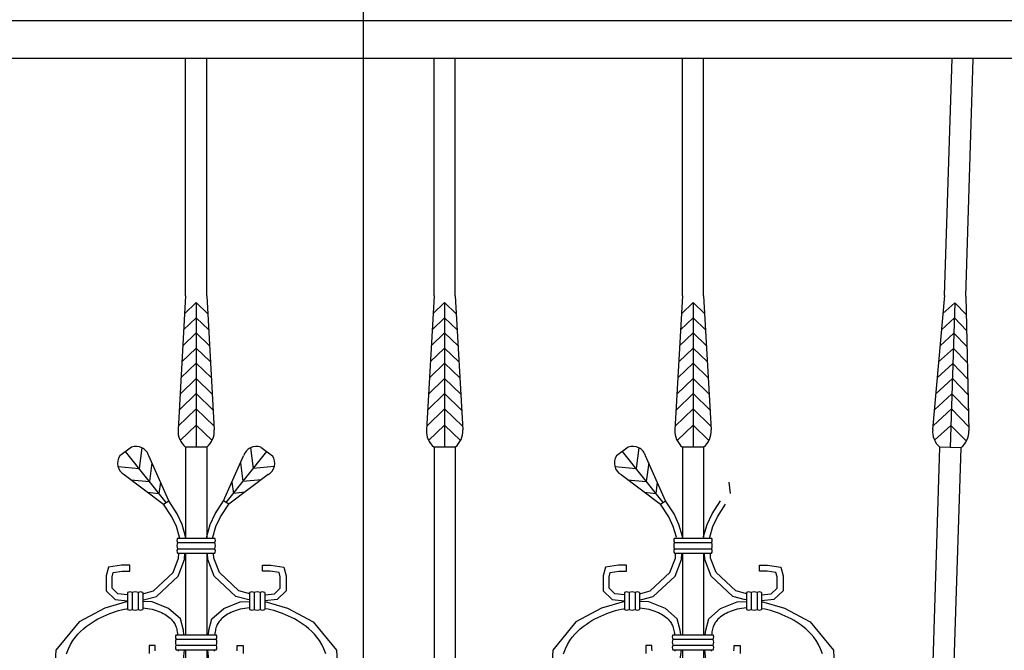
# Model space of a CAD drawing. Units: inches. Extents: x 2278 to 7495, y -71 to 1198.
# Tile 20 of 44: x 5007 to 5033, y 143 to 160. Entities that reach past the tile are written whole.
import ezdxf

# ---------------------------------------------------------------- set-up
doc = ezdxf.new("R2010")
doc.units = ezdxf.units.IN
doc.header["$MEASUREMENT"] = 0
doc.layers.add('A-ANNO-DIMS', color=2, linetype='Continuous', lineweight=18)
doc.layers.add('A-ELEV', color=7, linetype='Continuous', lineweight=25)
doc.styles.get("Standard").update_dxf_attribs({"font": 'arial.ttf'})
doc.dimstyles.get("Standard").update_dxf_attribs({"dimtxt": 6, "dimasz": 3, "dimexe": 0.18, "dimexo": 0.0625, "dimgap": 0.09, "dimtad": 0, "dimtih": 1, "dimtoh": 1, "dimdec": 0, "dimzin": 0, "dimdsep": 46, "dimlunit": 3, "dimtxsty": 'Standard', "dimblk": 'ARCHTICK', "dimcen": 0.09, "dimadec": 0, "dimazin": 0, "dimtfac": 1, "dimtdec": 0, "dimtofl": 0, "dimtmove": 0, "dimatfit": 3, "dimfxl": 1, "dimtolj": 1, "dimtzin": 0, "dimarcsym": 0})

# ---------------------------------------------------------------- blocks, each defined once
blk = doc.blocks.new('BALUSTER-ORNATE-A')
for p, q in [((3.585, 26.003), (3.585, 32.384)), ((4.155, 26.003), (4.155, 32.38)), ((3.585, 26.003), (3.383, 22.393)), ((4.155, 26.003), (4.357, 22.393)), ((3.558, 25.516), (3.87, 25.818)), ((3.87, 25.818), (3.87, 21.929)), ((4.182, 25.516), (3.87, 25.818)), ((3.533, 25.084), (3.87, 25.41)), ((4.207, 25.084), (3.87, 25.41)), ((3.509, 24.653), (3.87, 25.001)), ((4.231, 24.653), (3.87, 25.001)), ((3.485, 24.221), (3.87, 24.593)), ((4.255, 24.221), (3.87, 24.593)), ((3.461, 23.79), (3.87, 24.185)), ((4.279, 23.79), (3.87, 24.185)), ((3.437, 23.358), (3.87, 23.777)), ((4.303, 23.358), (3.87, 23.777)), ((3.413, 22.927), (3.87, 23.369)), ((4.327, 22.927), (3.87, 23.369)), ((3.388, 22.495), (3.87, 22.961)), ((4.352, 22.495), (3.87, 22.961)), ((3.442, 22.106), (3.87, 22.52)), ((4.299, 22.106), (3.87, 22.52)), ((2.128, 21.929), (1.813, 21.699)), ((3.063, 20.442), (1.97, 21.814)), ((2.412, 21.914), (2.339, 21.352)), ((3.585, 21.929), (3.585, 19.485)), ((4.155, 21.929), (3.585, 21.929)), ((4.155, 21.929), (4.155, 19.485)), ((4.677, 20.442), (5.77, 21.814)), ((5.328, 21.914), (5.401, 21.352)), ((5.612, 21.929), (5.927, 21.699)), ((3.131, 20.487), (2.594, 21.696)), ((2.678, 21.507), (2.613, 21.007)), ((4.609, 20.487), (5.146, 21.696)), ((5.062, 21.507), (5.127, 21.007)), ((1.774, 21.406), (2.339, 21.352)), ((1.936, 21.192), (2.995, 20.398)), ((5.804, 21.192), (4.745, 20.398)), ((5.966, 21.406), (5.401, 21.352)), ((2.111, 21.055), (2.613, 21.007)), ((2.907, 20.992), (2.868, 20.688)), ((4.833, 20.992), (4.872, 20.688)), ((5.629, 21.055), (5.127, 21.007)), ((2.562, 20.717), (2.868, 20.688)), ((5.178, 20.717), (4.872, 20.688)), ((2.995, 20.398), (3.131, 20.487)), ((3.217, 20.057), (2.995, 20.398)), ((3.36, 20.135), (3.131, 20.487)), ((4.38, 20.135), (4.609, 20.487)), ((4.523, 20.057), (4.745, 20.398)), ((4.745, 20.398), (4.609, 20.487)), ((3.49, 19.852), (3.36, 20.135)), ((4.25, 19.852), (4.38, 20.135)), ((3.337, 19.795), (3.217, 20.057)), ((4.403, 19.795), (4.523, 20.057)), ((3.421, 19.506), (3.337, 19.795)), ((3.585, 19.526), (3.49, 19.852)), ((4.155, 19.526), (4.25, 19.852)), ((4.319, 19.506), (4.403, 19.795)), ((3.37, 19.485), (4.37, 19.485)), ((3.37, 19.363), (4.37, 19.363)), ((3.42, 19.485), (3.421, 19.506)), ((3.583, 19.485), (3.585, 19.526)), ((4.157, 19.485), (4.155, 19.526)), ((4.32, 19.485), (4.319, 19.506)), ((3.37, 19.2), (4.37, 19.2)), ((3.37, 19.077), (4.37, 19.077)), ((3.396, 18.942), (3.402, 19.077)), ((3.558, 18.908), (3.565, 19.077)), ((3.585, 19.077), (3.585, 16.887)), ((4.155, 19.077), (4.155, 16.887)), ((4.182, 18.908), (4.175, 19.077)), ((4.344, 18.942), (4.338, 19.077)), ((3.247, 18.557), (3.396, 18.942)), ((3.385, 18.463), (3.558, 18.908)), ((4.355, 18.463), (4.182, 18.908)), ((4.493, 18.557), (4.344, 18.942)), ((1.513, 18.705), (1.449, 18.469)), ((1.866, 18.759), (1.513, 18.705)), ((1.612, 18.447), (1.642, 18.56)), ((1.642, 18.56), (1.879, 18.596)), ((2.084, 18.759), (1.866, 18.759)), ((1.879, 18.596), (2.084, 18.596)), ((2.084, 18.596), (2.084, 18.759)), ((2.719, 18.062), (3.247, 18.557)), ((5.021, 18.062), (4.493, 18.557)), ((5.656, 18.596), (5.656, 18.759)), ((5.656, 18.759), (5.874, 18.759)), ((5.861, 18.596), (5.656, 18.596)), ((6.098, 18.56), (5.861, 18.596)), ((5.874, 18.759), (6.227, 18.705)), ((6.128, 18.447), (6.098, 18.56)), ((6.227, 18.705), (6.291, 18.469)), ((1.449, 18.469), (1.449, 18.069)), ((1.612, 18.138), (1.612, 18.447)), ((2.801, 17.915), (3.385, 18.463)), ((4.939, 17.915), (4.355, 18.463)), ((6.128, 18.138), (6.128, 18.447)), ((6.291, 18.469), (6.291, 18.069)), ((1.449, 18.069), (1.694, 17.833)), ((1.767, 17.989), (1.612, 18.138)), ((2.026, 18.021), (2.026, 17.565)), ((2.148, 18.021), (2.148, 17.565)), ((2.311, 18.021), (2.311, 17.565)), ((2.434, 18.021), (2.434, 17.565)), ((2.462, 17.993), (2.719, 18.062)), ((5.278, 17.993), (5.021, 18.062)), ((5.306, 18.021), (5.306, 17.565)), ((5.429, 18.021), (5.429, 17.565)), ((5.592, 18.021), (5.592, 17.565)), ((5.714, 18.021), (5.714, 17.565)), ((5.973, 17.989), (6.128, 18.138)), ((6.291, 18.069), (6.046, 17.833)), ((2.026, 17.782), (1.412, 17.603)), ((1.694, 17.833), (2.026, 17.797)), ((2.026, 17.961), (1.767, 17.989)), ((2.434, 17.99), (2.462, 17.993)), ((2.434, 17.826), (2.492, 17.833)), ((2.683, 17.766), (2.434, 17.777)), ((2.492, 17.833), (2.801, 17.915)), ((3.128, 17.594), (2.683, 17.766)), ((4.612, 17.594), (5.057, 17.766)), ((5.248, 17.833), (4.939, 17.915)), ((5.057, 17.766), (5.306, 17.777)), ((5.306, 17.826), (5.248, 17.833)), ((5.306, 17.99), (5.278, 17.993)), ((5.714, 17.961), (5.973, 17.989)), ((6.046, 17.833), (5.714, 17.797)), ((5.714, 17.782), (6.328, 17.603)), ((1.412, 17.603), (0.722, 17.231)), ((1.549, 17.454), (1.627, 17.484)), ((1.627, 17.484), (1.705, 17.51)), ((1.705, 17.51), (1.782, 17.533)), ((1.782, 17.533), (1.858, 17.553)), ((1.858, 17.553), (1.933, 17.571)), ((1.933, 17.571), (2.007, 17.585)), ((2.007, 17.585), (2.026, 17.587)), ((2.434, 17.606), (2.499, 17.6)), ((2.499, 17.6), (2.563, 17.592)), ((2.563, 17.592), (2.624, 17.582)), ((2.624, 17.582), (2.683, 17.57)), ((2.683, 17.57), (2.739, 17.556)), ((2.739, 17.556), (2.792, 17.54)), ((2.792, 17.54), (2.843, 17.522)), ((2.843, 17.522), (2.891, 17.503)), ((2.891, 17.503), (2.937, 17.482)), ((2.937, 17.482), (2.981, 17.46)), ((3.446, 17.313), (3.128, 17.594)), ((4.294, 17.313), (4.612, 17.594)), ((4.803, 17.482), (4.759, 17.46)), ((4.849, 17.503), (4.803, 17.482)), ((4.897, 17.522), (4.849, 17.503)), ((4.948, 17.54), (4.897, 17.522)), ((5.001, 17.556), (4.948, 17.54)), ((5.057, 17.57), (5.001, 17.556)), ((5.116, 17.582), (5.057, 17.57)), ((5.177, 17.592), (5.116, 17.582)), ((5.241, 17.6), (5.177, 17.592)), ((5.306, 17.606), (5.241, 17.6)), ((5.733, 17.585), (5.714, 17.587)), ((5.807, 17.571), (5.733, 17.585)), ((5.882, 17.553), (5.807, 17.571)), ((5.958, 17.533), (5.882, 17.553)), ((6.035, 17.51), (5.958, 17.533)), ((6.113, 17.484), (6.035, 17.51)), ((6.191, 17.454), (6.113, 17.484)), ((6.328, 17.603), (7.018, 17.231)), ((0.722, 17.231), (0.096, 16.469)), ((0.993, 17.163), (1.071, 17.216)), ((1.071, 17.216), (1.15, 17.265)), ((1.15, 17.265), (1.23, 17.309)), ((1.23, 17.309), (1.309, 17.35)), ((1.309, 17.35), (1.389, 17.388)), ((1.389, 17.388), (1.469, 17.422)), ((1.469, 17.422), (1.549, 17.454)), ((2.981, 17.46), (3.024, 17.436)), ((3.024, 17.436), (3.064, 17.41)), ((3.064, 17.41), (3.102, 17.384)), ((3.102, 17.384), (3.138, 17.357)), ((3.138, 17.357), (3.171, 17.329)), ((3.171, 17.329), (3.201, 17.301)), ((3.201, 17.301), (3.228, 17.272)), ((3.228, 17.272), (3.252, 17.244)), ((3.252, 17.244), (3.272, 17.217)), ((3.272, 17.217), (3.288, 17.19)), ((3.528, 17.004), (3.446, 17.313)), ((4.212, 17.004), (4.294, 17.313)), ((4.468, 17.217), (4.452, 17.19)), ((4.489, 17.244), (4.468, 17.217)), ((4.512, 17.272), (4.489, 17.244)), ((4.539, 17.301), (4.512, 17.272)), ((4.569, 17.329), (4.539, 17.301)), ((4.602, 17.357), (4.569, 17.329)), ((4.638, 17.384), (4.602, 17.357)), ((4.676, 17.41), (4.638, 17.384)), ((4.716, 17.436), (4.676, 17.41)), ((4.759, 17.46), (4.716, 17.436)), ((6.271, 17.422), (6.191, 17.454)), ((6.351, 17.388), (6.271, 17.422)), ((6.431, 17.35), (6.351, 17.388)), ((6.51, 17.309), (6.431, 17.35)), ((6.59, 17.265), (6.51, 17.309)), ((6.669, 17.216), (6.59, 17.265)), ((6.747, 17.163), (6.669, 17.216)), ((7.018, 17.231), (7.644, 16.469)), ((0.692, 16.9), (0.764, 16.975)), ((0.764, 16.975), (0.839, 17.043)), ((0.839, 17.043), (0.916, 17.105)), ((0.916, 17.105), (0.993, 17.163)), ((3.288, 17.19), (3.303, 17.162)), ((3.303, 17.162), (3.316, 17.134)), ((3.316, 17.134), (3.327, 17.104)), ((3.327, 17.104), (3.337, 17.072)), ((3.337, 17.072), (3.346, 17.038)), ((3.346, 17.038), (3.354, 17.001)), ((3.354, 17.001), (3.361, 16.962)), ((3.361, 16.962), (3.368, 16.922)), ((3.542, 16.887), (3.528, 17.004)), ((4.198, 16.887), (4.212, 17.004)), ((4.379, 16.962), (4.372, 16.922)), ((4.386, 17.001), (4.379, 16.962)), ((4.394, 17.038), (4.386, 17.001)), ((4.403, 17.072), (4.394, 17.038)), ((4.413, 17.104), (4.403, 17.072)), ((4.424, 17.134), (4.413, 17.104)), ((4.437, 17.162), (4.424, 17.134)), ((4.452, 17.19), (4.437, 17.162)), ((6.824, 17.105), (6.747, 17.163)), ((6.901, 17.043), (6.824, 17.105)), ((6.976, 16.975), (6.901, 17.043)), ((7.048, 16.9), (6.976, 16.975)), ((0.495, 16.624), (0.557, 16.727)), ((0.557, 16.727), (0.623, 16.819)), ((0.623, 16.819), (0.692, 16.9)), ((3.329, 16.887), (4.411, 16.887)), ((3.329, 16.764), (4.411, 16.764)), ((3.368, 16.922), (3.374, 16.887)), ((4.372, 16.922), (4.366, 16.887)), ((7.117, 16.819), (7.048, 16.9)), ((7.183, 16.727), (7.117, 16.819)), ((7.245, 16.624), (7.183, 16.727)), ((0.096, 16.469), (0.025, 15.162)), ((0.386, 16.376), (0.438, 16.508)), ((0.438, 16.508), (0.495, 16.624)), ((2.764, 16.599), (2.602, 16.596)), ((2.602, 16.596), (2.602, 16.378)), ((2.766, 16.522), (2.764, 16.599)), ((2.769, 16.452), (2.766, 16.522)), ((3.329, 16.601), (4.411, 16.601)), ((3.329, 16.479), (4.411, 16.479)), ((3.388, 16.479), (3.383, 16.441)), ((3.528, 16.206), (3.557, 16.479)), ((3.585, 16.479), (3.585, 12.578)), ((4.155, 16.479), (4.155, 12.578)), ((4.212, 16.206), (4.183, 16.479)), ((4.352, 16.479), (4.357, 16.441)), ((4.971, 16.452), (4.974, 16.522)), ((4.974, 16.522), (4.976, 16.599)), ((4.976, 16.599), (5.138, 16.596)), ((5.138, 16.596), (5.138, 16.378)), ((7.302, 16.508), (7.245, 16.624)), ((7.354, 16.376), (7.302, 16.508)), ((7.644, 16.469), (7.715, 15.162))]:
    blk.add_line(p, q)
for centre, radius, start, end in [((3.929, 22.355), 0.547, 176.0178, 231.0717), ((3.811, 22.355), 0.547, 308.9283, 3.9822), ((2.253, 21.595), 0.356, 16.4025, 110.5063), ((5.487, 21.595), 0.356, 69.4937, 163.5975), ((2.111, 21.502), 0.356, 146.575, 240.6788), ((5.629, 21.502), 0.356, 299.3212, 33.425), ((3.475, 19.424), 0.121, 149.7768, 210.2232), ((3.563, 19.281), 0.209, 157.1017, 202.8983), ((4.265, 19.424), 0.121, 329.7768, 30.2232), ((4.177, 19.281), 0.209, 337.1017, 22.8983), ((3.475, 19.139), 0.121, 149.7768, 210.2232), ((4.265, 19.139), 0.121, 329.7768, 30.2232), ((2.087, 17.916), 0.121, 59.7768, 120.2232), ((2.23, 17.828), 0.209, 67.1017, 112.8983), ((2.373, 17.916), 0.121, 59.7768, 120.2232), ((5.368, 17.916), 0.121, 59.7768, 120.2232), ((5.51, 17.828), 0.209, 67.1017, 112.8983), ((5.653, 17.916), 0.121, 59.7768, 120.2232), ((2.087, 17.67), 0.121, 239.7768, 300.2232), ((2.23, 17.758), 0.209, 247.1017, 292.8983), ((2.373, 17.67), 0.121, 239.7768, 300.2232), ((5.368, 17.67), 0.121, 239.7768, 300.2232), ((5.51, 17.758), 0.209, 247.1017, 292.8983), ((5.653, 17.67), 0.121, 239.7768, 300.2232), ((3.434, 16.825), 0.121, 149.7768, 210.2232), ((3.522, 16.683), 0.209, 157.1017, 202.8983), ((4.306, 16.825), 0.121, 329.7768, 30.2232), ((4.218, 16.683), 0.209, 337.1017, 22.8983), ((3.434, 16.54), 0.121, 149.7768, 210.2232), ((4.306, 16.54), 0.121, 329.7768, 30.2232)]:
    blk.add_arc(centre, radius, start, end)
blk = doc.blocks.new('BALUSTER-ORNATE-B')
for p, q in [((3.585, 26.003), (3.585, 32.384)), ((4.155, 26.003), (4.155, 32.38)), ((3.585, 26.003), (3.383, 22.393)), ((4.155, 26.003), (4.358, 22.393)), ((3.558, 25.516), (3.87, 25.818)), ((3.87, 25.818), (3.87, 21.929)), ((4.183, 25.516), (3.87, 25.818)), ((3.534, 25.084), (3.87, 25.41)), ((4.207, 25.084), (3.87, 25.41)), ((3.51, 24.653), (3.87, 25.001)), ((4.231, 24.653), (3.87, 25.001)), ((3.485, 24.221), (3.87, 24.593)), ((4.255, 24.221), (3.87, 24.593)), ((3.461, 23.79), (3.87, 24.185)), ((4.279, 23.79), (3.87, 24.185)), ((3.437, 23.358), (3.87, 23.777)), ((4.304, 23.358), (3.87, 23.777)), ((3.413, 22.927), (3.87, 23.369)), ((4.328, 22.927), (3.87, 23.369)), ((3.389, 22.495), (3.87, 22.961)), ((4.352, 22.495), (3.87, 22.961)), ((3.442, 22.106), (3.87, 22.52)), ((4.299, 22.106), (3.87, 22.52)), ((2.128, 21.929), (1.814, 21.699)), ((3.063, 20.442), (1.971, 21.814)), ((2.412, 21.914), (2.339, 21.352)), ((3.585, 21.929), (3.585, 19.485)), ((4.155, 21.929), (3.585, 21.929)), ((4.155, 21.929), (4.155, 19.485)), ((3.132, 20.487), (2.595, 21.696)), ((2.679, 21.507), (2.614, 21.007)), ((1.774, 21.406), (2.339, 21.352)), ((1.936, 21.192), (2.995, 20.398)), ((2.112, 21.055), (2.614, 21.007)), ((2.907, 20.992), (2.868, 20.688)), ((4.833, 20.992), (4.873, 20.688)), ((2.563, 20.717), (2.868, 20.688)), ((2.995, 20.398), (3.132, 20.487)), ((3.217, 20.057), (2.995, 20.398)), ((3.36, 20.135), (3.132, 20.487)), ((4.381, 20.135), (4.609, 20.487)), ((4.524, 20.057), (4.746, 20.398)), ((3.49, 19.852), (3.36, 20.135)), ((4.251, 19.852), (4.381, 20.135)), ((3.337, 19.795), (3.217, 20.057)), ((4.404, 19.795), (4.524, 20.057)), ((3.421, 19.506), (3.337, 19.795)), ((3.585, 19.526), (3.49, 19.852)), ((4.155, 19.526), (4.251, 19.852)), ((4.319, 19.506), (4.404, 19.795)), ((3.37, 19.485), (4.37, 19.485)), ((3.37, 19.363), (4.37, 19.363)), ((3.42, 19.485), (3.421, 19.506)), ((3.583, 19.485), (3.585, 19.526)), ((4.157, 19.485), (4.155, 19.526)), ((4.32, 19.485), (4.319, 19.506)), ((3.37, 19.2), (4.37, 19.2)), ((3.37, 19.077), (4.37, 19.077)), ((3.396, 18.942), (3.402, 19.077)), ((3.558, 18.908), (3.565, 19.077)), ((3.585, 19.077), (3.585, 16.887)), ((4.155, 19.077), (4.155, 16.887)), ((4.183, 18.908), (4.175, 19.077)), ((4.344, 18.942), (4.338, 19.077)), ((3.247, 18.557), (3.396, 18.942)), ((3.386, 18.463), (3.558, 18.908)), ((4.355, 18.463), (4.183, 18.908)), ((4.494, 18.557), (4.344, 18.942)), ((1.513, 18.705), (1.449, 18.469)), ((1.867, 18.759), (1.513, 18.705)), ((1.612, 18.447), (1.643, 18.56)), ((1.643, 18.56), (1.879, 18.596)), ((2.084, 18.759), (1.867, 18.759)), ((1.879, 18.596), (2.084, 18.596)), ((2.084, 18.596), (2.084, 18.759)), ((2.72, 18.062), (3.247, 18.557)), ((5.021, 18.062), (4.494, 18.557)), ((5.656, 18.596), (5.656, 18.759)), ((5.656, 18.759), (5.874, 18.759)), ((5.861, 18.596), (5.656, 18.596)), ((6.098, 18.56), (5.861, 18.596)), ((5.874, 18.759), (6.228, 18.705)), ((6.128, 18.447), (6.098, 18.56)), ((6.228, 18.705), (6.291, 18.469)), ((1.449, 18.469), (1.449, 18.069)), ((1.612, 18.138), (1.612, 18.447)), ((2.801, 17.915), (3.386, 18.463)), ((4.939, 17.915), (4.355, 18.463)), ((6.128, 18.138), (6.128, 18.447)), ((6.291, 18.469), (6.291, 18.069)), ((1.449, 18.069), (1.694, 17.833)), ((1.767, 17.989), (1.612, 18.138)), ((2.027, 18.021), (2.027, 17.565)), ((2.149, 18.021), (2.149, 17.565)), ((2.312, 18.021), (2.312, 17.565)), ((2.434, 18.021), (2.434, 17.565)), ((2.462, 17.993), (2.72, 18.062)), ((5.279, 17.993), (5.021, 18.062)), ((5.307, 18.021), (5.307, 17.565)), ((5.429, 18.021), (5.429, 17.565)), ((5.592, 18.021), (5.592, 17.565)), ((5.714, 18.021), (5.714, 17.565)), ((5.973, 17.989), (6.128, 18.138)), ((6.291, 18.069), (6.046, 17.833)), ((2.027, 17.782), (1.412, 17.603)), ((1.694, 17.833), (2.027, 17.797)), ((2.027, 17.961), (1.767, 17.989)), ((2.434, 17.99), (2.462, 17.993)), ((2.434, 17.826), (2.493, 17.833)), ((2.684, 17.766), (2.434, 17.777)), ((2.493, 17.833), (2.801, 17.915)), ((3.128, 17.594), (2.684, 17.766)), ((4.612, 17.594), (5.057, 17.766)), ((5.248, 17.833), (4.939, 17.915)), ((5.057, 17.766), (5.307, 17.777)), ((5.307, 17.826), (5.248, 17.833)), ((5.307, 17.99), (5.279, 17.993)), ((5.714, 17.961), (5.973, 17.989)), ((6.046, 17.833), (5.714, 17.797)), ((5.714, 17.782), (6.328, 17.603)), ((1.412, 17.603), (0.722, 17.231)), ((1.549, 17.454), (1.628, 17.484)), ((1.628, 17.484), (1.705, 17.51)), ((1.705, 17.51), (1.782, 17.533)), ((1.782, 17.533), (1.858, 17.553)), ((1.858, 17.553), (1.933, 17.571)), ((1.933, 17.571), (2.008, 17.585)), ((2.008, 17.585), (2.027, 17.587)), ((2.434, 17.606), (2.5, 17.6)), ((2.5, 17.6), (2.563, 17.592)), ((2.563, 17.592), (2.625, 17.582)), ((2.625, 17.582), (2.683, 17.57)), ((2.683, 17.57), (2.739, 17.556)), ((2.739, 17.556), (2.792, 17.54)), ((2.792, 17.54), (2.843, 17.522)), ((2.843, 17.522), (2.891, 17.503)), ((2.891, 17.503), (2.937, 17.482)), ((2.937, 17.482), (2.982, 17.46)), ((3.446, 17.313), (3.128, 17.594)), ((4.294, 17.313), (4.612, 17.594)), ((4.803, 17.482), (4.759, 17.46)), ((4.849, 17.503), (4.803, 17.482)), ((4.898, 17.522), (4.849, 17.503)), ((4.948, 17.54), (4.898, 17.522)), ((5.002, 17.556), (4.948, 17.54)), ((5.057, 17.57), (5.002, 17.556)), ((5.116, 17.582), (5.057, 17.57)), ((5.177, 17.592), (5.116, 17.582)), ((5.241, 17.6), (5.177, 17.592)), ((5.307, 17.606), (5.241, 17.6)), ((5.733, 17.585), (5.714, 17.587)), ((5.807, 17.571), (5.733, 17.585)), ((5.882, 17.553), (5.807, 17.571)), ((5.958, 17.533), (5.882, 17.553)), ((6.035, 17.51), (5.958, 17.533)), ((6.113, 17.484), (6.035, 17.51)), ((6.192, 17.454), (6.113, 17.484)), ((6.328, 17.603), (7.018, 17.231)), ((0.722, 17.231), (0.096, 16.469)), ((0.994, 17.163), (1.072, 17.216)), ((1.072, 17.216), (1.151, 17.265)), ((1.151, 17.265), (1.23, 17.309)), ((1.23, 17.309), (1.309, 17.35)), ((1.309, 17.35), (1.389, 17.388)), ((1.389, 17.388), (1.469, 17.422)), ((1.469, 17.422), (1.549, 17.454)), ((2.982, 17.46), (3.024, 17.436)), ((3.024, 17.436), (3.064, 17.41)), ((3.064, 17.41), (3.103, 17.384)), ((3.103, 17.384), (3.138, 17.357)), ((3.138, 17.357), (3.171, 17.329)), ((3.171, 17.329), (3.201, 17.301)), ((3.201, 17.301), (3.228, 17.272)), ((3.228, 17.272), (3.252, 17.244)), ((3.252, 17.244), (3.272, 17.217)), ((3.272, 17.217), (3.289, 17.19)), ((3.528, 17.004), (3.446, 17.313)), ((4.213, 17.004), (4.294, 17.313)), ((4.469, 17.217), (4.452, 17.19)), ((4.489, 17.244), (4.469, 17.217)), ((4.512, 17.272), (4.489, 17.244)), ((4.539, 17.301), (4.512, 17.272)), ((4.569, 17.329), (4.539, 17.301)), ((4.602, 17.357), (4.569, 17.329)), ((4.638, 17.384), (4.602, 17.357)), ((4.676, 17.41), (4.638, 17.384)), ((4.717, 17.436), (4.676, 17.41)), ((4.759, 17.46), (4.717, 17.436)), ((6.271, 17.422), (6.192, 17.454)), ((6.351, 17.388), (6.271, 17.422)), ((6.431, 17.35), (6.351, 17.388)), ((6.511, 17.309), (6.431, 17.35)), ((6.59, 17.265), (6.511, 17.309)), ((6.669, 17.216), (6.59, 17.265)), ((6.747, 17.163), (6.669, 17.216)), ((7.018, 17.231), (7.645, 16.469)), ((0.692, 16.9), (0.765, 16.975)), ((0.765, 16.975), (0.839, 17.043)), ((0.839, 17.043), (0.916, 17.105)), ((0.916, 17.105), (0.994, 17.163)), ((3.289, 17.19), (3.303, 17.162)), ((3.303, 17.162), (3.316, 17.134)), ((3.316, 17.134), (3.327, 17.104)), ((3.327, 17.104), (3.337, 17.072)), ((3.337, 17.072), (3.346, 17.038)), ((3.346, 17.038), (3.354, 17.001)), ((3.354, 17.001), (3.362, 16.962)), ((3.362, 16.962), (3.369, 16.922)), ((3.542, 16.887), (3.528, 17.004)), ((4.199, 16.887), (4.213, 17.004)), ((4.379, 16.962), (4.372, 16.922)), ((4.387, 17.001), (4.379, 16.962)), ((4.395, 17.038), (4.387, 17.001)), ((4.404, 17.072), (4.395, 17.038)), ((4.413, 17.104), (4.404, 17.072)), ((4.425, 17.134), (4.413, 17.104)), ((4.437, 17.162), (4.425, 17.134)), ((4.452, 17.19), (4.437, 17.162)), ((6.825, 17.105), (6.747, 17.163)), ((6.901, 17.043), (6.825, 17.105)), ((6.976, 16.975), (6.901, 17.043)), ((7.048, 16.9), (6.976, 16.975)), ((0.496, 16.624), (0.557, 16.727)), ((0.557, 16.727), (0.623, 16.819)), ((0.623, 16.819), (0.692, 16.9)), ((3.33, 16.887), (4.411, 16.887)), ((3.33, 16.764), (4.411, 16.764)), ((3.369, 16.922), (3.374, 16.887)), ((4.372, 16.922), (4.366, 16.887)), ((7.117, 16.819), (7.048, 16.9)), ((7.183, 16.727), (7.117, 16.819)), ((7.245, 16.624), (7.183, 16.727)), ((0.096, 16.469), (0.025, 15.162)), ((0.386, 16.376), (0.438, 16.508)), ((0.438, 16.508), (0.496, 16.624)), ((2.765, 16.599), (2.602, 16.596)), ((2.602, 16.596), (2.602, 16.378)), ((2.766, 16.522), (2.765, 16.599)), ((2.769, 16.452), (2.766, 16.522)), ((3.33, 16.601), (4.411, 16.601)), ((3.33, 16.479), (4.411, 16.479)), ((3.388, 16.479), (3.384, 16.441)), ((3.528, 16.206), (3.558, 16.479)), ((3.585, 16.479), (3.585, 12.578)), ((4.155, 16.479), (4.155, 12.578)), ((4.213, 16.206), (4.183, 16.479)), ((4.352, 16.479), (4.357, 16.441)), ((4.971, 16.452), (4.975, 16.522)), ((4.975, 16.522), (4.976, 16.599)), ((4.976, 16.599), (5.139, 16.596)), ((5.139, 16.596), (5.139, 16.378)), ((7.302, 16.508), (7.245, 16.624)), ((7.354, 16.376), (7.302, 16.508)), ((7.645, 16.469), (7.715, 15.162))]:
    blk.add_line(p, q)
for centre, radius, start, end in [((3.929, 22.355), 0.547, 176.0178, 231.0717), ((3.811, 22.355), 0.547, 308.9283, 3.9822), ((2.253, 21.595), 0.356, 16.4025, 110.5063), ((2.111, 21.502), 0.356, 146.575, 240.6788), ((3.475, 19.424), 0.121, 149.7768, 210.2232), ((3.563, 19.281), 0.209, 157.1017, 202.8983), ((4.265, 19.424), 0.121, 329.7768, 30.2232), ((4.177, 19.281), 0.209, 337.1017, 22.8983), ((3.475, 19.139), 0.121, 149.7768, 210.2232), ((4.265, 19.139), 0.121, 329.7768, 30.2232), ((2.088, 17.916), 0.121, 59.7768, 120.2232), ((2.23, 17.828), 0.209, 67.1017, 112.8983), ((2.373, 17.916), 0.121, 59.7768, 120.2232), ((5.368, 17.916), 0.121, 59.7768, 120.2232), ((5.51, 17.828), 0.209, 67.1017, 112.8983), ((5.653, 17.916), 0.121, 59.7768, 120.2232), ((2.088, 17.67), 0.121, 239.7768, 300.2232), ((2.23, 17.758), 0.209, 247.1017, 292.8983), ((2.373, 17.67), 0.121, 239.7768, 300.2232), ((5.368, 17.67), 0.121, 239.7768, 300.2232), ((5.51, 17.758), 0.209, 247.1017, 292.8983), ((5.653, 17.67), 0.121, 239.7768, 300.2232), ((3.434, 16.825), 0.121, 149.7768, 210.2232), ((3.522, 16.683), 0.209, 157.1017, 202.8983), ((4.306, 16.825), 0.121, 329.7768, 30.2232), ((4.218, 16.683), 0.209, 337.1017, 22.8983), ((3.434, 16.54), 0.121, 149.7768, 210.2232), ((4.306, 16.54), 0.121, 329.7768, 30.2232)]:
    blk.add_arc(centre, radius, start, end)
blk = doc.blocks.new('RAIL-BAR-A')
for p, q in [((0.202, 26.003), (0.202, 32.38)), ((0.773, 26.003), (0.773, 32.38)), ((0.202, 26.003), (0, 22.393)), ((0.773, 26.003), (0.975, 22.393)), ((0.175, 25.516), (0.488, 25.818)), ((0.488, 25.818), (0.488, 21.929)), ((0.8, 25.516), (0.488, 25.818)), ((0.151, 25.084), (0.488, 25.41)), ((0.824, 25.084), (0.488, 25.41)), ((0.127, 24.653), (0.488, 25.001)), ((0.848, 24.653), (0.488, 25.001)), ((0.103, 24.221), (0.488, 24.593)), ((0.873, 24.221), (0.488, 24.593)), ((0.079, 23.79), (0.488, 24.185)), ((0.897, 23.79), (0.488, 24.185)), ((0.054, 23.358), (0.488, 23.777)), ((0.921, 23.358), (0.488, 23.777)), ((0.03, 22.927), (0.488, 23.369)), ((0.945, 22.927), (0.488, 23.369)), ((0.006, 22.495), (0.488, 22.961)), ((0.969, 22.495), (0.488, 22.961)), ((0.059, 22.106), (0.488, 22.52)), ((0.916, 22.106), (0.488, 22.52)), ((0.202, 21.929), (0.202, 7.128)), ((0.773, 21.929), (0.202, 21.929)), ((0.773, 21.929), (0.773, 7.128))]:
    blk.add_line(p, q)
for centre, start, end in [((0.546, 22.355), 176.0178, 231.0717), ((0.429, 22.355), 308.9283, 3.9822)]:
    blk.add_arc(centre, 0.547, start, end)
blk = doc.blocks.new('RAIL-BAR-C')
for p, q in [((0.203, 26.003), (0.203, 32.38)), ((0.773, 32.38), (0.203, 32.38)), ((0.773, 26.003), (0.773, 32.38)), ((0.203, 26.003), (0, 22.393)), ((0.773, 26.003), (0.975, 22.393)), ((0.175, 25.516), (0.488, 25.818)), ((0.488, 25.818), (0.488, 21.929)), ((0.8, 25.516), (0.488, 25.818)), ((0.151, 25.084), (0.488, 25.41)), ((0.824, 25.084), (0.488, 25.41)), ((0.127, 24.653), (0.488, 25.001)), ((0.848, 24.653), (0.488, 25.001)), ((0.103, 24.221), (0.488, 24.593)), ((0.873, 24.221), (0.488, 24.593)), ((0.079, 23.79), (0.488, 24.185)), ((0.897, 23.79), (0.488, 24.185)), ((0.054, 23.358), (0.488, 23.777)), ((0.921, 23.358), (0.488, 23.777)), ((0.03, 22.927), (0.488, 23.369)), ((0.945, 22.927), (0.488, 23.369)), ((0.006, 22.495), (0.488, 22.961)), ((0.969, 22.495), (0.488, 22.961)), ((0.059, 22.106), (0.488, 22.52)), ((0.916, 22.106), (0.488, 22.52)), ((0.203, 21.929), (0.203, 7.128)), ((0.773, 21.929), (0.203, 21.929)), ((0.773, 21.929), (0.773, 7.128))]:
    blk.add_line(p, q)
for centre, start, end in [((0.547, 22.355), 176.0178, 231.0717), ((0.429, 22.355), 308.9283, 3.9822)]:
    blk.add_arc(centre, 0.547, start, end)
blk = doc.blocks.new('_ArchTick')
at = {"color": 0, "linetype": 'ByBlock', "const_width": 0.15}
blk.add_lwpolyline([(-0.5, -0.5), (0.5, 0.5)], dxfattribs=at)
blk = doc.blocks.new('*D123')
at = {"layer": 'A-ANNO-DIMS', "color": 0, "lineweight": -2, "transparency": 16777216}
for p, q in [((4736.95, 340.157), (4736.95, -23.427)), ((5145.676, -1.81), (5145.676, -23.427)), ((4736.95, -23.247), (4923.929, -23.247)), ((5145.676, -23.247), (4958.697, -23.247))]:
    blk.add_line(p, q, dxfattribs=at)
at = {"layer": 'Defpoints', "color": 0, "transparency": 16777216}
for p in [(4736.95, 340.219), (5145.676, -1.747), (5145.676, -23.247)]:
    blk.add_point(p, dxfattribs=at)
at = {"layer": 'A-ANNO-DIMS', "color": 0, "lineweight": -2, "transparency": 16777216, "xscale": 3, "yscale": 3, "zscale": 3, "rotation": 180}
blk.add_blockref('_ArchTick', (4736.95, -23.247), dxfattribs=at)
at = {"layer": 'A-ANNO-DIMS', "color": 0, "lineweight": -2, "transparency": 16777216, "xscale": 3, "yscale": 3, "zscale": 3}
blk.add_blockref('_ArchTick', (5145.676, -23.247), dxfattribs=at)
at = {"layer": 'A-ANNO-DIMS', "color": 0, "transparency": 16777216, "insert": (4941.313, -23.247), "char_height": 6, "attachment_point": 5}
blk.add_mtext('\\A1;34\'-0 1/2"', dxfattribs=at)
blk = doc.blocks.new('*D129')
at = {"layer": 'A-ANNO-DIMS', "color": 0, "lineweight": -2, "transparency": 16777216}
for p, q in [((4970.676, 60.779), (4970.676, 361.899)), ((4970.676, 361.719), (4978.373, 361.719)), ((5016.176, 361.719), (5008.479, 361.719)), ((5016.176, 99.315), (5016.176, 361.899))]:
    blk.add_line(p, q, dxfattribs=at)
at = {"layer": 'Defpoints', "color": 0, "transparency": 16777216}
for p in [(5016.176, 361.719), (5016.176, 99.253), (4970.676, 60.717)]:
    blk.add_point(p, dxfattribs=at)
at = {"layer": 'A-ANNO-DIMS', "color": 0, "lineweight": -2, "transparency": 16777216, "xscale": 3, "yscale": 3, "zscale": 3, "rotation": 180}
blk.add_blockref('_ArchTick', (4970.676, 361.719), dxfattribs=at)
at = {"layer": 'A-ANNO-DIMS', "color": 0, "lineweight": -2, "transparency": 16777216, "xscale": 3, "yscale": 3, "zscale": 3}
blk.add_blockref('_ArchTick', (5016.176, 361.719), dxfattribs=at)
at = {"layer": 'A-ANNO-DIMS', "color": 0, "transparency": 16777216, "insert": (4993.426, 361.719), "char_height": 6, "attachment_point": 5}
blk.add_mtext('\\A1;3\'-9 1/2"', dxfattribs=at)
blk = doc.blocks.new('*D130')
at = {"layer": 'A-ANNO-DIMS', "color": 0, "lineweight": -2, "transparency": 16777216}
for p, q in [((5016.176, 99.315), (5016.176, 361.899)), ((5016.176, 361.719), (5048.095, 361.719)), ((5096.176, 361.719), (5064.257, 361.719)), ((5096.176, 99.315), (5096.176, 361.899))]:
    blk.add_line(p, q, dxfattribs=at)
at = {"layer": 'Defpoints', "color": 0, "transparency": 16777216}
for p in [(5096.176, 361.719), (5016.176, 99.253), (5096.176, 99.253)]:
    blk.add_point(p, dxfattribs=at)
at = {"layer": 'A-ANNO-DIMS', "color": 0, "lineweight": -2, "transparency": 16777216, "xscale": 3, "yscale": 3, "zscale": 3, "rotation": 180}
blk.add_blockref('_ArchTick', (5016.176, 361.719), dxfattribs=at)
at = {"layer": 'A-ANNO-DIMS', "color": 0, "lineweight": -2, "transparency": 16777216, "xscale": 3, "yscale": 3, "zscale": 3}
blk.add_blockref('_ArchTick', (5096.176, 361.719), dxfattribs=at)
at = {"layer": 'A-ANNO-DIMS', "color": 0, "transparency": 16777216, "insert": (5056.176, 361.719), "char_height": 6, "attachment_point": 5}
blk.add_mtext('\\A1;6\'-8"', dxfattribs=at)

msp = doc.modelspace()

# ---------------------------------------------------------------- linework, layer by layer
at = {"layer": 'A-ELEV'}
for p, q in [((5065.039, 160.198), (4971.673, 160.198)), ((5065.039, 159.179), (4971.673, 159.179))]:
    msp.add_line(p, q, dxfattribs=at)

# ---------------------------------------------------------------- block references
for name, p in [('BALUSTER-ORNATE-A', (5007.805, 126.799)), ('RAIL-BAR-C', (5017.868, 126.799)), ('BALUSTER-ORNATE-B', (5021.166, 126.799))]:
    msp.add_blockref(name, p, dxfattribs=at)
at = {"layer": 'A-ELEV', "rotation": 358.1636620681507}
msp.add_blockref('RAIL-BAR-A', (5030.762, 126.822), dxfattribs=at)

# ---------------------------------------------------------------- dimensions: what is measured, and where the dimension line sits
at = {"layer": 'A-ANNO-DIMS'}
for base, p1, p2, picture, middle in [((5016.176, 361.719), (4970.676, 60.717), (5016.176, 99.253), '*D129', (4993.426, 361.719)), ((5096.176, 361.719), (5016.176, 99.253), (5096.176, 99.253), '*D130', (5056.176, 361.719)), ((5145.676, -23.247), (4736.95, 340.219), (5145.676, -1.747), '*D123', (4941.313, -23.247))]:
    dim = msp.add_linear_dim(base=base, p1=p1, p2=p2, dimstyle='Standard', override={"dimdec": 1, "dimlfac": 1, "dimrnd": 0, "dimzin": 1, "dimdsep": 46, "dimlunit": 4, "dimfrac": 2}, dxfattribs=at)
    dim.commit()
    dim.dimension.update_dxf_attribs({"geometry": picture, "text_midpoint": middle})

doc.saveas('drawing.dxf')
